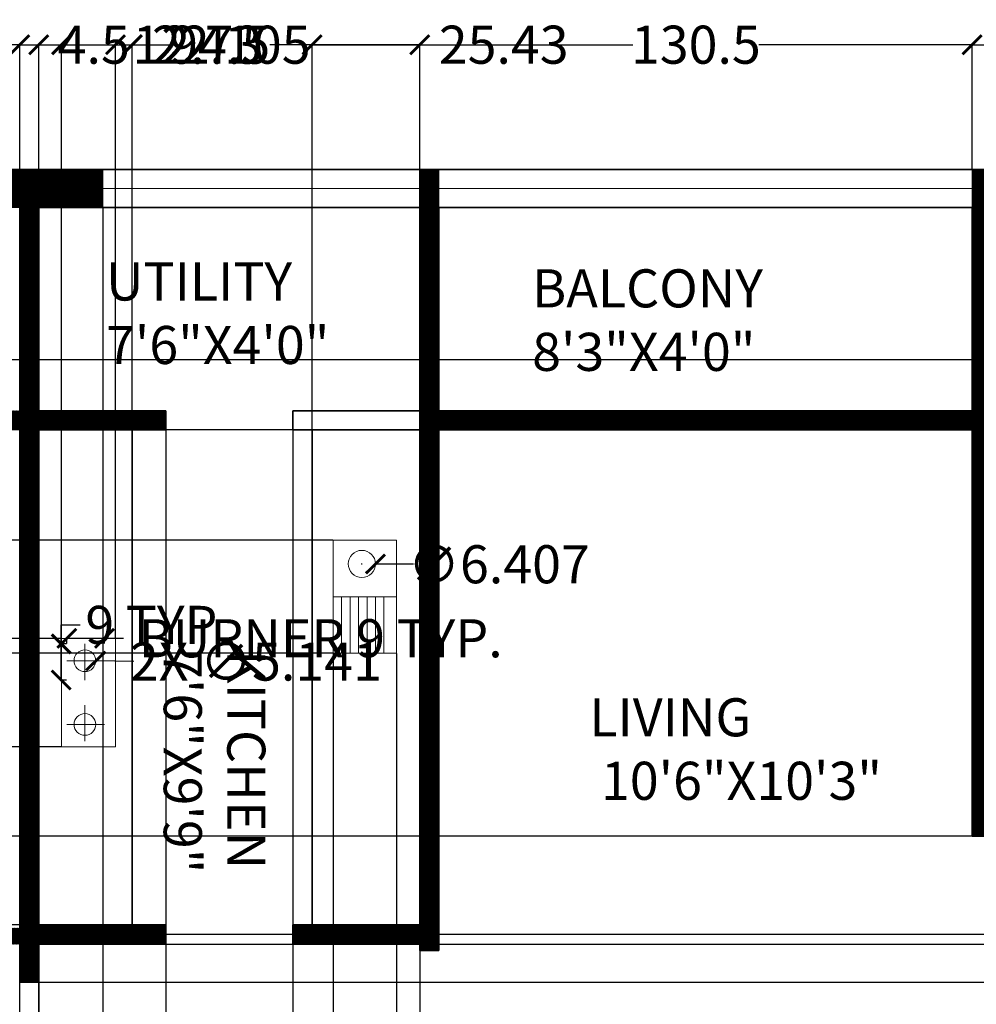
# Model space of a CAD drawing. Units: inches. Extents: x -9 to 675, y 146 to 566.
# Tile 3 of 4: x 192 to 418, y 334 to 566. Entities that reach past the tile are written whole.
import ezdxf

# ---------------------------------------------------------------- set-up
doc = ezdxf.new("R2010")
doc.units = ezdxf.units.IN
doc.header["$MEASUREMENT"] = 0
for name, color, linetype, lineweight in [('A-ANNO-DIMS', 2, 'Continuous', 18), ('A-AREA-IDEN', 7, 'Continuous', 18), ('A-EQPM', 8, 'Continuous', 18), ('A-FLOR-CASE', 8, 'Continuous', 25), ('A-FLOR-FIXT', 9, 'Continuous', 18), ('A-GLAZ', 4, 'Continuous', 18), ('A-WALL', 7, 'Continuous', 35), ('A-WALL-PATT', 252, 'Continuous', 13)]:
    doc.layers.add(name, color=color, linetype=linetype, lineweight=lineweight)
doc.styles.get("Standard").update_dxf_attribs({"font": 'arial.ttf'})
doc.dimstyles.get("Standard").update_dxf_attribs({"dimtxt": 9, "dimasz": 4.5, "dimexe": 0.18, "dimexo": 0.0625, "dimgap": 0.09, "dimtad": 0, "dimtih": 1, "dimtoh": 1, "dimdec": 1, "dimzin": 0, "dimdsep": 46, "dimlunit": 4, "dimtxsty": 'Standard', "dimblk": 'ARCHTICK', "dimcen": 0.09, "dimadec": 0, "dimazin": 0, "dimtfac": 1, "dimtdec": 1, "dimtofl": 0, "dimtmove": 0, "dimatfit": 3, "dimfxl": 1, "dimtolj": 1, "dimtzin": 0, "dimarcsym": 0})

# ---------------------------------------------------------------- blocks, each defined once
blk = doc.blocks.new('COOKTOP-BURNER')
for p, q in [((4.27, 4.56), (4.27, 8.54)), ((4.27, 8.54), (4.27, 4.56)), ((4.27, 4.56), (0, 4.56)), ((4.27, 4.56), (8.88, 4.56)), ((8.88, 4.56), (4.27, 4.56)), ((4.27, 4.56), (4.27, 0)), ((4.27, 0), (4.27, 4.56))]:
    blk.add_line(p, q)
blk.add_circle((4.27, 4.56), 2.57)
blk = doc.blocks.new('_ArchTick')
at = {"color": 0, "linetype": 'ByBlock', "const_width": 0.15}
blk.add_lwpolyline([(-0.5, -0.5), (0.5, 0.5)], dxfattribs=at)
blk = doc.blocks.new('*D6')
at = {"layer": 'A-ANNO-DIMS', "color": 0, "lineweight": -2, "transparency": 16777216}
for p, q in [((203.45, 418.99), (203.45, 420.43)), ((203.45, 420.25), (212.33, 420.25)), ((212.33, 418.99), (212.33, 420.43)), ((212.33, 420.25), (216.83, 420.25))]:
    blk.add_line(p, q, dxfattribs=at)
at = {"layer": 'Defpoints', "color": 0, "transparency": 16777216}
for p in [(203.45, 418.92), (212.33, 420.25), (212.33, 418.92)]:
    blk.add_point(p, dxfattribs=at)
at = {"layer": 'A-ANNO-DIMS', "color": 0, "lineweight": -2, "transparency": 16777216, "xscale": 4.5, "yscale": 4.5, "zscale": 4.5, "rotation": 180}
blk.add_blockref('_ArchTick', (203.45, 420.25), dxfattribs=at)
at = {"layer": 'A-ANNO-DIMS', "color": 0, "lineweight": -2, "transparency": 16777216, "xscale": 4.5, "yscale": 4.5, "zscale": 4.5}
blk.add_blockref('_ArchTick', (212.33, 420.25), dxfattribs=at)
at = {"layer": 'A-ANNO-DIMS', "color": 0, "transparency": 16777216, "insert": (263.42, 420.25), "char_height": 9, "attachment_point": 5}
blk.add_mtext('\\A1;BURNER 9 TYP.', dxfattribs=at)
blk = doc.blocks.new('*D7')
at = {"layer": 'A-ANNO-DIMS', "color": 0, "lineweight": -2, "transparency": 16777216}
for p, q in [((202.12, 418.92), (202.12, 423.42)), ((202.12, 423.42), (206.62, 423.42)), ((203.39, 418.92), (201.94, 418.92)), ((202.12, 410.39), (202.12, 418.92)), ((203.39, 410.39), (201.94, 410.39))]:
    blk.add_line(p, q, dxfattribs=at)
at = {"layer": 'Defpoints', "color": 0, "transparency": 16777216}
for p in [(202.12, 418.92), (203.45, 418.92), (203.45, 410.39)]:
    blk.add_point(p, dxfattribs=at)
at = {"layer": 'A-ANNO-DIMS', "color": 0, "lineweight": -2, "transparency": 16777216, "xscale": 4.5, "yscale": 4.5, "zscale": 4.5}
for p, rotation in [((202.12, 418.92), 90), ((202.12, 410.39), 270)]:
    blk.add_blockref('_ArchTick', p, dxfattribs=dict(at, rotation=rotation))
at = {"layer": 'A-ANNO-DIMS', "color": 0, "transparency": 16777216, "insert": (225.12, 423.42), "char_height": 9, "attachment_point": 5}
blk.add_mtext('\\A1;9 TYP.', dxfattribs=at)
blk = doc.blocks.new('*D11')
at = {"layer": 'A-ANNO-DIMS', "color": 0, "lineweight": -2, "transparency": 16777216}
for p, q in [((121.3, 531.07), (121.3, 560.69)), ((192.3, 522.07), (192.3, 560.69)), ((121.3, 560.51), (151.17, 560.51)), ((192.3, 560.51), (162.43, 560.51))]:
    blk.add_line(p, q, dxfattribs=at)
at = {"layer": 'Defpoints', "color": 0, "transparency": 16777216}
for p in [(192.3, 560.51), (121.3, 531.01), (192.3, 522.01)]:
    blk.add_point(p, dxfattribs=at)
at = {"layer": 'A-ANNO-DIMS', "color": 0, "lineweight": -2, "transparency": 16777216, "xscale": 4.5, "yscale": 4.5, "zscale": 4.5, "rotation": 180}
blk.add_blockref('_ArchTick', (121.3, 560.51), dxfattribs=at)
at = {"layer": 'A-ANNO-DIMS', "color": 0, "lineweight": -2, "transparency": 16777216, "xscale": 4.5, "yscale": 4.5, "zscale": 4.5}
blk.add_blockref('_ArchTick', (192.3, 560.51), dxfattribs=at)
at = {"layer": 'A-ANNO-DIMS', "color": 0, "transparency": 16777216, "insert": (156.8, 560.51), "char_height": 9, "attachment_point": 5}
blk.add_mtext('\\A1;71', dxfattribs=at)
blk = doc.blocks.new('*D12')
at = {"layer": 'A-ANNO-DIMS', "color": 0, "lineweight": -2, "transparency": 16777216}
for p, q in [((192.3, 522.07), (192.3, 560.69)), ((286.8, 531.07), (286.8, 560.69)), ((192.3, 560.51), (227.74, 560.51)), ((286.8, 560.51), (251.37, 560.51))]:
    blk.add_line(p, q, dxfattribs=at)
at = {"layer": 'Defpoints', "color": 0, "transparency": 16777216}
for p in [(286.8, 560.51), (286.8, 531.01), (192.3, 522.01)]:
    blk.add_point(p, dxfattribs=at)
at = {"layer": 'A-ANNO-DIMS', "color": 0, "lineweight": -2, "transparency": 16777216, "xscale": 4.5, "yscale": 4.5, "zscale": 4.5, "rotation": 180}
blk.add_blockref('_ArchTick', (192.3, 560.51), dxfattribs=at)
at = {"layer": 'A-ANNO-DIMS', "color": 0, "lineweight": -2, "transparency": 16777216, "xscale": 4.5, "yscale": 4.5, "zscale": 4.5}
blk.add_blockref('_ArchTick', (286.8, 560.51), dxfattribs=at)
at = {"layer": 'A-ANNO-DIMS', "color": 0, "transparency": 16777216, "insert": (239.55, 560.51), "char_height": 9, "attachment_point": 5}
blk.add_mtext('\\A1;94.5', dxfattribs=at)
blk = doc.blocks.new('*D13')
at = {"layer": 'A-ANNO-DIMS', "color": 0, "lineweight": -2, "transparency": 16777216}
for p, q in [((286.8, 531.07), (286.8, 560.69)), ((417.3, 531.07), (417.3, 560.69)), ((286.8, 560.51), (337.17, 560.51)), ((417.3, 560.51), (366.94, 560.51))]:
    blk.add_line(p, q, dxfattribs=at)
at = {"layer": 'Defpoints', "color": 0, "transparency": 16777216}
for p in [(417.3, 560.51), (286.8, 531.01), (417.3, 531.01)]:
    blk.add_point(p, dxfattribs=at)
at = {"layer": 'A-ANNO-DIMS', "color": 0, "lineweight": -2, "transparency": 16777216, "xscale": 4.5, "yscale": 4.5, "zscale": 4.5, "rotation": 180}
blk.add_blockref('_ArchTick', (286.8, 560.51), dxfattribs=at)
at = {"layer": 'A-ANNO-DIMS', "color": 0, "lineweight": -2, "transparency": 16777216, "xscale": 4.5, "yscale": 4.5, "zscale": 4.5}
blk.add_blockref('_ArchTick', (417.3, 560.51), dxfattribs=at)
at = {"layer": 'A-ANNO-DIMS', "color": 0, "transparency": 16777216, "insert": (352.05, 560.51), "char_height": 9, "attachment_point": 5}
blk.add_mtext('\\A1;130.5', dxfattribs=at)
blk = doc.blocks.new('*D14')
at = {"layer": 'A-ANNO-DIMS', "color": 0, "lineweight": -2, "transparency": 16777216}
for p, q in [((417.3, 531.07), (417.3, 560.69)), ((550.8, 531.07), (550.8, 560.69)), ((417.3, 560.51), (469.17, 560.51)), ((550.8, 560.51), (498.94, 560.51))]:
    blk.add_line(p, q, dxfattribs=at)
at = {"layer": 'Defpoints', "color": 0, "transparency": 16777216}
for p in [(550.8, 560.51), (417.3, 531.01), (550.8, 531.01)]:
    blk.add_point(p, dxfattribs=at)
at = {"layer": 'A-ANNO-DIMS', "color": 0, "lineweight": -2, "transparency": 16777216, "xscale": 4.5, "yscale": 4.5, "zscale": 4.5, "rotation": 180}
blk.add_blockref('_ArchTick', (417.3, 560.51), dxfattribs=at)
at = {"layer": 'A-ANNO-DIMS', "color": 0, "lineweight": -2, "transparency": 16777216, "xscale": 4.5, "yscale": 4.5, "zscale": 4.5}
blk.add_blockref('_ArchTick', (550.8, 560.51), dxfattribs=at)
at = {"layer": 'A-ANNO-DIMS', "color": 0, "transparency": 16777216, "insert": (484.05, 560.51), "char_height": 9, "attachment_point": 5}
blk.add_mtext('\\A1;133.5', dxfattribs=at)
blk = doc.blocks.new('*D26')
at = {"layer": 'A-ANNO-DIMS', "color": 0, "lineweight": -2, "transparency": 16777216}
for p, q in [((211.96, 521.95), (211.96, 151.83)), ((286.8, 521.95), (286.8, 151.83)), ((211.96, 152.01), (234.16, 152.01)), ((286.8, 152.01), (264.6, 152.01))]:
    blk.add_line(p, q, dxfattribs=at)
at = {"layer": 'Defpoints', "color": 0, "transparency": 16777216}
for p in [(211.96, 522.01), (286.8, 522.01), (286.8, 152.01)]:
    blk.add_point(p, dxfattribs=at)
at = {"layer": 'A-ANNO-DIMS', "color": 0, "lineweight": -2, "transparency": 16777216, "xscale": 4.5, "yscale": 4.5, "zscale": 4.5, "rotation": 180}
blk.add_blockref('_ArchTick', (211.96, 152.01), dxfattribs=at)
at = {"layer": 'A-ANNO-DIMS', "color": 0, "lineweight": -2, "transparency": 16777216, "xscale": 4.5, "yscale": 4.5, "zscale": 4.5}
blk.add_blockref('_ArchTick', (286.8, 152.01), dxfattribs=at)
at = {"layer": 'A-ANNO-DIMS', "color": 0, "transparency": 16777216, "insert": (249.38, 152.01), "char_height": 9, "attachment_point": 5}
blk.add_mtext('\\A1;74.84', dxfattribs=at)
blk = doc.blocks.new('*D28')
at = {"layer": 'A-ANNO-DIMS', "color": 0, "lineweight": -2, "transparency": 16777216}
for p, q in [((196.8, 469.45), (196.8, 151.83)), ((226.8, 469.45), (226.8, 151.83)), ((196.8, 152.01), (205.28, 152.01)), ((226.8, 152.01), (218.32, 152.01))]:
    blk.add_line(p, q, dxfattribs=at)
at = {"layer": 'Defpoints', "color": 0, "transparency": 16777216}
for p in [(196.8, 469.51), (226.8, 469.51), (226.8, 152.01)]:
    blk.add_point(p, dxfattribs=at)
at = {"layer": 'A-ANNO-DIMS', "color": 0, "lineweight": -2, "transparency": 16777216, "xscale": 4.5, "yscale": 4.5, "zscale": 4.5, "rotation": 180}
blk.add_blockref('_ArchTick', (196.8, 152.01), dxfattribs=at)
at = {"layer": 'A-ANNO-DIMS', "color": 0, "lineweight": -2, "transparency": 16777216, "xscale": 4.5, "yscale": 4.5, "zscale": 4.5}
blk.add_blockref('_ArchTick', (226.8, 152.01), dxfattribs=at)
at = {"layer": 'A-ANNO-DIMS', "color": 0, "transparency": 16777216, "insert": (211.8, 152.01), "char_height": 9, "attachment_point": 5}
blk.add_mtext('\\A1;30', dxfattribs=at)
blk = doc.blocks.new('*D29')
at = {"layer": 'A-ANNO-DIMS', "color": 0, "lineweight": -2, "transparency": 16777216}
for p, q in [((226.8, 469.45), (226.8, 151.83)), ((256.8, 469.45), (256.8, 151.83)), ((226.8, 152.01), (235.28, 152.01)), ((256.8, 152.01), (248.32, 152.01))]:
    blk.add_line(p, q, dxfattribs=at)
at = {"layer": 'Defpoints', "color": 0, "transparency": 16777216}
for p in [(226.8, 469.51), (256.8, 469.51), (256.8, 152.01)]:
    blk.add_point(p, dxfattribs=at)
at = {"layer": 'A-ANNO-DIMS', "color": 0, "lineweight": -2, "transparency": 16777216, "xscale": 4.5, "yscale": 4.5, "zscale": 4.5, "rotation": 180}
blk.add_blockref('_ArchTick', (226.8, 152.01), dxfattribs=at)
at = {"layer": 'A-ANNO-DIMS', "color": 0, "lineweight": -2, "transparency": 16777216, "xscale": 4.5, "yscale": 4.5, "zscale": 4.5}
blk.add_blockref('_ArchTick', (256.8, 152.01), dxfattribs=at)
at = {"layer": 'A-ANNO-DIMS', "color": 0, "transparency": 16777216, "insert": (241.8, 152.01), "char_height": 9, "attachment_point": 5}
blk.add_mtext('\\A1;30', dxfattribs=at)
blk = doc.blocks.new('*D30')
at = {"layer": 'A-ANNO-DIMS', "color": 0, "lineweight": -2, "transparency": 16777216}
for p, q in [((226.8, 347.95), (226.8, 151.83)), ((256.8, 347.95), (256.8, 151.83)), ((226.8, 152.01), (235.28, 152.01)), ((256.8, 152.01), (248.32, 152.01))]:
    blk.add_line(p, q, dxfattribs=at)
at = {"layer": 'Defpoints', "color": 0, "transparency": 16777216}
for p in [(226.8, 348.01), (256.8, 348.01), (256.8, 152.01)]:
    blk.add_point(p, dxfattribs=at)
at = {"layer": 'A-ANNO-DIMS', "color": 0, "lineweight": -2, "transparency": 16777216, "xscale": 4.5, "yscale": 4.5, "zscale": 4.5, "rotation": 180}
blk.add_blockref('_ArchTick', (226.8, 152.01), dxfattribs=at)
at = {"layer": 'A-ANNO-DIMS', "color": 0, "lineweight": -2, "transparency": 16777216, "xscale": 4.5, "yscale": 4.5, "zscale": 4.5}
blk.add_blockref('_ArchTick', (256.8, 152.01), dxfattribs=at)
at = {"layer": 'A-ANNO-DIMS', "color": 0, "transparency": 16777216, "insert": (241.8, 152.01), "char_height": 9, "attachment_point": 5}
blk.add_mtext('\\A1;30', dxfattribs=at)
blk = doc.blocks.new('*D33')
at = {"layer": 'A-ANNO-DIMS', "color": 0, "lineweight": -2, "transparency": 16777216}
for p, q in [((655.8, 348.01), (655.8, 352.51)), ((655.8, 352.51), (660.3, 352.51)), ((196.87, 348.01), (655.98, 348.01)), ((655.8, 339.01), (655.8, 348.01)), ((196.87, 339.01), (655.98, 339.01))]:
    blk.add_line(p, q, dxfattribs=at)
at = {"layer": 'Defpoints', "color": 0, "transparency": 16777216}
for p in [(196.8, 348.01), (655.8, 348.01), (196.8, 339.01)]:
    blk.add_point(p, dxfattribs=at)
at = {"layer": 'A-ANNO-DIMS', "color": 0, "lineweight": -2, "transparency": 16777216, "xscale": 4.5, "yscale": 4.5, "zscale": 4.5}
for p, rotation in [((655.8, 348.01), 90), ((655.8, 339.01), 270)]:
    blk.add_blockref('_ArchTick', p, dxfattribs=dict(at, rotation=rotation))
at = {"layer": 'A-ANNO-DIMS', "color": 0, "transparency": 16777216, "insert": (663.35, 352.51), "char_height": 9, "attachment_point": 5}
blk.add_mtext('\\A1;9', dxfattribs=at)
blk = doc.blocks.new('*D34')
at = {"layer": 'A-ANNO-DIMS', "color": 0, "lineweight": -2, "transparency": 16777216}
for p, q in [((196.87, 339.01), (655.98, 339.01)), ((655.8, 339.01), (655.8, 322.62)), ((655.8, 297.01), (655.8, 313.4)), ((196.87, 297.01), (655.98, 297.01))]:
    blk.add_line(p, q, dxfattribs=at)
at = {"layer": 'Defpoints', "color": 0, "transparency": 16777216}
for p in [(196.8, 339.01), (655.8, 339.01), (196.8, 297.01)]:
    blk.add_point(p, dxfattribs=at)
at = {"layer": 'A-ANNO-DIMS', "color": 0, "lineweight": -2, "transparency": 16777216, "xscale": 4.5, "yscale": 4.5, "zscale": 4.5}
for p, rotation in [((655.8, 339.01), 90), ((655.8, 297.01), 270)]:
    blk.add_blockref('_ArchTick', p, dxfattribs=dict(at, rotation=rotation))
at = {"layer": 'A-ANNO-DIMS', "color": 0, "transparency": 16777216, "insert": (655.8, 318.01), "char_height": 9, "attachment_point": 5}
blk.add_mtext('\\A1;42', dxfattribs=at)
blk = doc.blocks.new('*D42')
at = {"layer": 'A-ANNO-DIMS', "color": 0, "lineweight": -2, "transparency": 16777216}
for p, q in [((196.8, 352.57), (196.8, 560.69)), ((218.91, 352.57), (218.91, 560.69)), ((196.8, 560.51), (218.91, 560.51)), ((218.91, 560.51), (223.41, 560.51))]:
    blk.add_line(p, q, dxfattribs=at)
at = {"layer": 'Defpoints', "color": 0, "transparency": 16777216}
for p in [(218.91, 560.51), (196.8, 352.51), (218.91, 352.51)]:
    blk.add_point(p, dxfattribs=at)
at = {"layer": 'A-ANNO-DIMS', "color": 0, "lineweight": -2, "transparency": 16777216, "xscale": 4.5, "yscale": 4.5, "zscale": 4.5, "rotation": 180}
blk.add_blockref('_ArchTick', (196.8, 560.51), dxfattribs=at)
at = {"layer": 'A-ANNO-DIMS', "color": 0, "lineweight": -2, "transparency": 16777216, "xscale": 4.5, "yscale": 4.5, "zscale": 4.5}
blk.add_blockref('_ArchTick', (218.91, 560.51), dxfattribs=at)
at = {"layer": 'A-ANNO-DIMS', "color": 0, "transparency": 16777216, "insert": (242.29, 560.51), "char_height": 9, "attachment_point": 5}
blk.add_mtext('\\A1;22.105', dxfattribs=at)
blk = doc.blocks.new('*D43')
at = {"layer": 'A-ANNO-DIMS', "color": 0, "lineweight": -2, "transparency": 16777216}
for p, q in [((261.37, 352.57), (261.37, 560.69)), ((286.8, 352.57), (286.8, 560.69)), ((261.37, 560.51), (286.8, 560.51)), ((286.8, 560.51), (291.3, 560.51))]:
    blk.add_line(p, q, dxfattribs=at)
at = {"layer": 'Defpoints', "color": 0, "transparency": 16777216}
for p in [(286.8, 560.51), (261.37, 352.51), (286.8, 352.51)]:
    blk.add_point(p, dxfattribs=at)
at = {"layer": 'A-ANNO-DIMS', "color": 0, "lineweight": -2, "transparency": 16777216, "xscale": 4.5, "yscale": 4.5, "zscale": 4.5, "rotation": 180}
blk.add_blockref('_ArchTick', (261.37, 560.51), dxfattribs=at)
at = {"layer": 'A-ANNO-DIMS', "color": 0, "lineweight": -2, "transparency": 16777216, "xscale": 4.5, "yscale": 4.5, "zscale": 4.5}
blk.add_blockref('_ArchTick', (286.8, 560.51), dxfattribs=at)
at = {"layer": 'A-ANNO-DIMS', "color": 0, "transparency": 16777216, "insert": (306.65, 560.51), "char_height": 9, "attachment_point": 5}
blk.add_mtext('\\A1;25.43', dxfattribs=at)
blk = doc.blocks.new('*D46')
at = {"layer": 'A-ANNO-DIMS', "color": 0, "lineweight": -2, "transparency": 16777216}
for p, q in [((435.74, 522.01), (9.62, 522.01)), ((9.8, 522.01), (9.8, 508.7)), ((9.8, 486.01), (9.8, 499.32)), ((445.74, 486.01), (9.62, 486.01))]:
    blk.add_line(p, q, dxfattribs=at)
at = {"layer": 'Defpoints', "color": 0, "transparency": 16777216}
for p in [(435.8, 522.01), (9.8, 486.01), (445.8, 486.01)]:
    blk.add_point(p, dxfattribs=at)
at = {"layer": 'A-ANNO-DIMS', "color": 0, "lineweight": -2, "transparency": 16777216, "xscale": 4.5, "yscale": 4.5, "zscale": 4.5}
for p, rotation in [((9.8, 522.01), 90), ((9.8, 486.01), 270)]:
    blk.add_blockref('_ArchTick', p, dxfattribs=dict(at, rotation=rotation))
at = {"layer": 'A-ANNO-DIMS', "color": 0, "transparency": 16777216, "insert": (9.8, 504.01), "char_height": 9, "attachment_point": 5}
blk.add_mtext('\\A1;36', dxfattribs=at)
blk = doc.blocks.new('*D47')
at = {"layer": 'A-ANNO-DIMS', "color": 0, "lineweight": -2, "transparency": 16777216}
for p, q in [((617.24, 373.51), (9.62, 373.51)), ((9.8, 373.51), (9.8, 366.56)), ((9.8, 350.24), (9.8, 357.19)), ((602.52, 350.24), (9.62, 350.24))]:
    blk.add_line(p, q, dxfattribs=at)
at = {"layer": 'Defpoints', "color": 0, "transparency": 16777216}
for p in [(617.3, 373.51), (9.8, 350.24), (602.59, 350.24)]:
    blk.add_point(p, dxfattribs=at)
at = {"layer": 'A-ANNO-DIMS', "color": 0, "lineweight": -2, "transparency": 16777216, "xscale": 4.5, "yscale": 4.5, "zscale": 4.5}
for p, rotation in [((9.8, 373.51), 90), ((9.8, 350.24), 270)]:
    blk.add_blockref('_ArchTick', p, dxfattribs=dict(at, rotation=rotation))
at = {"layer": 'A-ANNO-DIMS', "color": 0, "transparency": 16777216, "insert": (9.8, 361.87), "char_height": 9, "attachment_point": 5}
blk.add_mtext('\\A1;23.27', dxfattribs=at)
blk = doc.blocks.new('*D50')
at = {"layer": 'A-ANNO-DIMS', "color": 0, "lineweight": -2, "transparency": 16777216}
for p, q in [((192.3, 297.07), (192.3, 560.69)), ((196.8, 297.07), (196.8, 560.69)), ((192.3, 560.51), (196.8, 560.51)), ((196.8, 560.51), (201.3, 560.51))]:
    blk.add_line(p, q, dxfattribs=at)
at = {"layer": 'Defpoints', "color": 0, "transparency": 16777216}
for p in [(196.8, 560.51), (192.3, 297.01), (196.8, 297.01)]:
    blk.add_point(p, dxfattribs=at)
at = {"layer": 'A-ANNO-DIMS', "color": 0, "lineweight": -2, "transparency": 16777216, "xscale": 4.5, "yscale": 4.5, "zscale": 4.5, "rotation": 180}
blk.add_blockref('_ArchTick', (192.3, 560.51), dxfattribs=at)
at = {"layer": 'A-ANNO-DIMS', "color": 0, "lineweight": -2, "transparency": 16777216, "xscale": 4.5, "yscale": 4.5, "zscale": 4.5}
blk.add_blockref('_ArchTick', (196.8, 560.51), dxfattribs=at)
at = {"layer": 'A-ANNO-DIMS', "color": 0, "transparency": 16777216, "insert": (209.8, 560.51), "char_height": 9, "attachment_point": 5}
blk.add_mtext('\\A1;4.5', dxfattribs=at)
blk = doc.blocks.new('*D51')
at = {"layer": 'A-ANNO-DIMS', "color": 0, "lineweight": -2, "transparency": 16777216}
for p, q in [((266.36, 416.64), (266.36, 151.83)), ((281.29, 416.64), (281.29, 151.83)), ((266.36, 152.01), (281.29, 152.01)), ((281.29, 152.01), (285.79, 152.01))]:
    blk.add_line(p, q, dxfattribs=at)
at = {"layer": 'Defpoints', "color": 0, "transparency": 16777216}
for p in [(266.36, 416.7), (281.29, 416.7), (281.29, 152.01)]:
    blk.add_point(p, dxfattribs=at)
at = {"layer": 'A-ANNO-DIMS', "color": 0, "lineweight": -2, "transparency": 16777216, "xscale": 4.5, "yscale": 4.5, "zscale": 4.5, "rotation": 180}
blk.add_blockref('_ArchTick', (266.36, 152.01), dxfattribs=at)
at = {"layer": 'A-ANNO-DIMS', "color": 0, "lineweight": -2, "transparency": 16777216, "xscale": 4.5, "yscale": 4.5, "zscale": 4.5}
blk.add_blockref('_ArchTick', (281.29, 152.01), dxfattribs=at)
at = {"layer": 'A-ANNO-DIMS', "color": 0, "transparency": 16777216, "insert": (300.65, 152.01), "char_height": 9, "attachment_point": 5}
blk.add_mtext('\\A1;14.93', dxfattribs=at)
blk = doc.blocks.new('*D52')
at = {"layer": 'A-ANNO-DIMS', "color": 0, "lineweight": -2, "transparency": 16777216}
for p, q in [((266.3, 443.4), (9.62, 443.4)), ((9.8, 443.4), (9.8, 434.74)), ((9.8, 416.7), (9.8, 425.37)), ((266.3, 416.7), (9.62, 416.7))]:
    blk.add_line(p, q, dxfattribs=at)
at = {"layer": 'Defpoints', "color": 0, "transparency": 16777216}
for p in [(9.8, 443.4), (266.36, 443.4), (266.36, 416.7)]:
    blk.add_point(p, dxfattribs=at)
at = {"layer": 'A-ANNO-DIMS', "color": 0, "lineweight": -2, "transparency": 16777216, "xscale": 4.5, "yscale": 4.5, "zscale": 4.5}
for p, rotation in [((9.8, 443.4), 90), ((9.8, 416.7), 270)]:
    blk.add_blockref('_ArchTick', p, dxfattribs=dict(at, rotation=rotation))
at = {"layer": 'A-ANNO-DIMS', "color": 0, "transparency": 16777216, "insert": (9.8, 430.05), "char_height": 9, "attachment_point": 5}
blk.add_mtext('\\A1;26.705', dxfattribs=at)
blk = doc.blocks.new('*D53')
at = {"layer": 'A-ANNO-DIMS', "color": 0, "lineweight": -2, "transparency": 16777216}
for p, q in [((261.31, 469.51), (9.62, 469.51)), ((9.8, 469.51), (9.8, 461.14)), ((9.8, 443.4), (9.8, 451.77)), ((266.3, 443.4), (9.62, 443.4))]:
    blk.add_line(p, q, dxfattribs=at)
at = {"layer": 'Defpoints', "color": 0, "transparency": 16777216}
for p in [(261.37, 469.51), (9.8, 443.4), (266.36, 443.4)]:
    blk.add_point(p, dxfattribs=at)
at = {"layer": 'A-ANNO-DIMS', "color": 0, "lineweight": -2, "transparency": 16777216, "xscale": 4.5, "yscale": 4.5, "zscale": 4.5}
for p, rotation in [((9.8, 469.51), 90), ((9.8, 443.4), 270)]:
    blk.add_blockref('_ArchTick', p, dxfattribs=dict(at, rotation=rotation))
at = {"layer": 'A-ANNO-DIMS', "color": 0, "transparency": 16777216, "insert": (9.8, 456.46), "char_height": 9, "attachment_point": 5}
blk.add_mtext('\\A1;26.106', dxfattribs=at)
blk = doc.blocks.new('*D54')
at = {"layer": 'A-ANNO-DIMS', "color": 0, "lineweight": -2, "transparency": 16777216}
for p, q in [((202.21, 420.27), (202.21, 560.69)), ((214.94, 420.27), (214.94, 560.69)), ((202.21, 560.51), (214.94, 560.51)), ((214.94, 560.51), (219.44, 560.51))]:
    blk.add_line(p, q, dxfattribs=at)
at = {"layer": 'Defpoints', "color": 0, "transparency": 16777216}
for p in [(214.94, 560.51), (202.21, 420.2), (214.94, 420.2)]:
    blk.add_point(p, dxfattribs=at)
at = {"layer": 'A-ANNO-DIMS', "color": 0, "lineweight": -2, "transparency": 16777216, "xscale": 4.5, "yscale": 4.5, "zscale": 4.5, "rotation": 180}
blk.add_blockref('_ArchTick', (202.21, 560.51), dxfattribs=at)
at = {"layer": 'A-ANNO-DIMS', "color": 0, "lineweight": -2, "transparency": 16777216, "xscale": 4.5, "yscale": 4.5, "zscale": 4.5}
blk.add_blockref('_ArchTick', (214.94, 560.51), dxfattribs=at)
at = {"layer": 'A-ANNO-DIMS', "color": 0, "transparency": 16777216, "insert": (234.3, 560.51), "char_height": 9, "attachment_point": 5}
blk.add_mtext('\\A1;12.73', dxfattribs=at)
blk = doc.blocks.new('*D55')
at = {"layer": 'A-ANNO-DIMS', "color": 0, "lineweight": -2, "transparency": 16777216}
for p, q in [((202.15, 420.2), (9.62, 420.2)), ((9.8, 420.2), (9.8, 412.11)), ((9.8, 394.64), (9.8, 402.74)), ((202.15, 394.64), (9.62, 394.64))]:
    blk.add_line(p, q, dxfattribs=at)
at = {"layer": 'Defpoints', "color": 0, "transparency": 16777216}
for p in [(9.8, 420.2), (202.21, 420.2), (202.21, 394.64)]:
    blk.add_point(p, dxfattribs=at)
at = {"layer": 'A-ANNO-DIMS', "color": 0, "lineweight": -2, "transparency": 16777216, "xscale": 4.5, "yscale": 4.5, "zscale": 4.5}
for p, rotation in [((9.8, 420.2), 90), ((9.8, 394.64), 270)]:
    blk.add_blockref('_ArchTick', p, dxfattribs=dict(at, rotation=rotation))
at = {"layer": 'A-ANNO-DIMS', "color": 0, "transparency": 16777216, "insert": (9.8, 407.42), "char_height": 9, "attachment_point": 5}
blk.add_mtext('\\A1;25.57', dxfattribs=at)
blk = doc.blocks.new('*D56')
at = {"layer": 'A-ANNO-DIMS', "color": 0, "lineweight": -2, "transparency": 16777216}
for p, q in [((202.15, 394.64), (9.62, 394.64)), ((9.8, 394.64), (9.8, 378.26)), ((9.8, 352.51), (9.8, 368.89)), ((196.74, 352.51), (9.62, 352.51))]:
    blk.add_line(p, q, dxfattribs=at)
at = {"layer": 'Defpoints', "color": 0, "transparency": 16777216}
for p in [(9.8, 394.64), (202.21, 394.64), (196.8, 352.51)]:
    blk.add_point(p, dxfattribs=at)
at = {"layer": 'A-ANNO-DIMS', "color": 0, "lineweight": -2, "transparency": 16777216, "xscale": 4.5, "yscale": 4.5, "zscale": 4.5}
for p, rotation in [((9.8, 394.64), 90), ((9.8, 352.51), 270)]:
    blk.add_blockref('_ArchTick', p, dxfattribs=dict(at, rotation=rotation))
at = {"layer": 'A-ANNO-DIMS', "color": 0, "transparency": 16777216, "insert": (9.8, 373.57), "char_height": 9, "attachment_point": 5}
blk.add_mtext('\\A1;42.126', dxfattribs=at)
blk = doc.blocks.new('*D58')
at = {"layer": 'A-ANNO-DIMS', "color": 0, "lineweight": -2, "transparency": 16777216}
for p, q in [((273.06, 437.82), (273.24, 437.82)), ((273.15, 437.73), (273.15, 437.91)), ((285.35, 437.74), (276.35, 437.8))]:
    blk.add_line(p, q, dxfattribs=at)
at = {"layer": 'Defpoints', "color": 0, "transparency": 16777216}
for p in [(269.95, 437.84), (276.35, 437.8)]:
    blk.add_point(p, dxfattribs=at)
at = {"layer": 'A-ANNO-DIMS', "color": 0, "lineweight": -2, "transparency": 16777216, "xscale": 4.5, "yscale": 4.5, "zscale": 4.5, "rotation": 179.6150108270535}
blk.add_blockref('_ArchTick', (276.35, 437.8), dxfattribs=at)
at = {"layer": 'A-ANNO-DIMS', "color": 0, "transparency": 16777216, "insert": (305.52, 437.74), "char_height": 9, "attachment_point": 5}
blk.add_mtext('\\A1;∅6.407', dxfattribs=at)
blk = doc.blocks.new('*D59')
at = {"layer": 'A-ANNO-DIMS', "color": 0, "lineweight": -2, "transparency": 16777216}
for p, q in [((207.63, 414.94), (207.81, 414.94)), ((207.72, 414.85), (207.72, 415.03)), ((219.29, 414.75), (210.29, 414.9))]:
    blk.add_line(p, q, dxfattribs=at)
at = {"layer": 'Defpoints', "color": 0, "transparency": 16777216}
for p in [(205.15, 414.99), (210.29, 414.9)]:
    blk.add_point(p, dxfattribs=at)
at = {"layer": 'A-ANNO-DIMS', "color": 0, "lineweight": -2, "transparency": 16777216, "xscale": 4.5, "yscale": 4.5, "zscale": 4.5, "rotation": 179.0165020891146}
blk.add_blockref('_ArchTick', (210.29, 414.9), dxfattribs=at)
at = {"layer": 'A-ANNO-DIMS', "color": 0, "transparency": 16777216, "insert": (248.1, 414.75), "char_height": 9, "attachment_point": 5}
blk.add_mtext('\\A1;2X ∅5.141', dxfattribs=at)

msp = doc.modelspace()

# ---------------------------------------------------------------- hatches: boundary and pattern name
at = {"layer": 'A-WALL-PATT'}
h = msp.add_hatch(dxfattribs=at)
h.set_pattern_fill('ANSI31', color=256)
h.paths.add_polyline_path([(361.8026, 244.5097), (357.3026, 244.5097), (357.3026, 228.4917), (286.8026, 228.4917), (196.8026, 228.4917), (196.8026, 297.0097), (192.3026, 297.0097), (192.3026, 190.5097), (196.8026, 190.5097), (196.8026, 219.4917), (286.8026, 219.4917), (357.3026, 219.4917), (357.3026, 217.5097), (357.3026, 214.9917), (361.8026, 214.9917), (361.8026, 217.5097)])
h.paths.add_polyline_path([(532.6092, 217.5097), (541.8026, 217.5097), (550.8026, 217.5097), (626.3026, 217.5097), (626.3026, 373.5097), (626.3026, 378.0097), (617.3026, 378.0097), (617.3026, 373.5097), (617.3026, 226.5097), (550.8026, 226.5097), (541.8026, 226.5097), (488.3026, 226.5097), (488.3026, 331.0097), (483.8026, 331.0097), (474.8026, 331.0097), (474.8026, 326.5097), (483.8026, 326.5097), (483.8026, 226.5097), (421.8026, 226.5097), (421.8026, 326.5097), (444.8026, 326.5097), (444.8026, 331.0097), (421.8026, 331.0097), (417.3026, 331.0097), (417.3026, 217.5097), (417.3026, 190.5097), (387.6027, 190.5097), (361.8026, 190.5097), (361.8026, 195.0097), (357.3026, 195.0097), (357.3026, 190.5097), (357.3026, 181.5097), (387.6027, 181.5097), (421.8026, 181.5097), (532.6092, 181.5097)])
h.paths.add_polyline_path([(421.8026, 190.5097), (421.8026, 217.5097), (523.6092, 217.5097), (523.6092, 190.5097)], flags=16)
h.paths.add_polyline_path([(550.8026, 378.0097), (550.8026, 531.0097), (525.3955, 531.0097), (525.3955, 522.0097), (541.8026, 522.0097), (541.8026, 378.0097), (472.8026, 378.0097), (472.8026, 373.5097), (483.8026, 373.5097), (488.3026, 373.5097), (541.8026, 373.5097), (550.8026, 373.5097)])
h.paths.add_polyline_path([(130.3026, 469.5097), (146.3026, 469.5097), (146.3026, 474.0097), (130.3026, 474.0097), (130.3026, 522.0097), (143.3026, 522.0097), (143.3026, 531.0097), (121.3026, 531.0097), (121.3026, 351.7597), (121.3026, 348.0097), (130.3026, 348.0097), (139.3026, 348.0097), (139.3026, 351.7597), (130.3026, 351.7597)])
h.paths.add_polyline_path([(211.9624, 531.0097), (179.3026, 531.0097), (179.3026, 522.0097), (192.3026, 522.0097), (192.3026, 474.0097), (176.3026, 474.0097), (176.3026, 469.5097), (192.3026, 469.5097), (192.3026, 351.7597), (169.3026, 351.7597), (169.3026, 348.0097), (192.3026, 348.0097), (192.3026, 339.0097), (196.8026, 339.0097), (196.8026, 348.0097), (226.8026, 348.0097), (226.8026, 352.5097), (196.8026, 352.5097), (196.8026, 469.5097), (226.8026, 469.5097), (226.8026, 474.0097), (196.8026, 474.0097), (196.8026, 522.0097), (211.9624, 522.0097)])
h.paths.add_polyline_path([(291.3026, 522.0097), (291.3026, 531.0097), (286.8026, 531.0097), (286.8026, 522.0097), (286.8026, 352.5097), (256.8026, 352.5097), (256.8026, 348.0097), (286.8026, 348.0097), (286.8026, 346.5097), (291.3026, 346.5097)])
h.paths.add_polyline_path([(417.3026, 474.0097), (291.3026, 474.0097), (291.3026, 469.5097), (417.3026, 469.5097)])
h.paths.add_polyline_path([(421.8026, 522.0097), (435.8002, 522.0097), (435.8002, 531.0097), (417.3026, 531.0097), (417.3026, 522.0097), (417.3026, 373.5097), (421.8026, 373.5097), (430.8026, 373.5097), (430.8026, 378.0097), (421.8026, 378.0097)])
h.paths.add_polyline_path([(48.3026, 348.0097), (48.3026, 351.7597), (39.3026, 351.7597), (39.3026, 348.0097), (39.3026, 181.5097), (121.3026, 181.5097), (196.8026, 181.5097), (196.8026, 190.5097), (192.3026, 190.5097), (121.3026, 190.5097), (48.3026, 190.5097)])

# ---------------------------------------------------------------- linework, layer by layer
at = {"layer": 'A-EQPM'}
for p, q in [((202.2142, 420.205), (214.9443, 420.205)), ((202.2142, 394.6354), (202.2142, 420.205)), ((214.9443, 420.205), (214.9443, 394.6354)), ((214.9443, 394.6354), (202.2142, 394.6354))]:
    msp.add_line(p, q, dxfattribs=at)
at = {"layer": 'A-FLOR-CASE'}
for p, q in [((218.9076, 469.5097), (218.9076, 352.5097)), ((261.3749, 469.5097), (261.3749, 352.5097))]:
    msp.add_line(p, q, dxfattribs=at)
at = {"layer": 'A-FLOR-FIXT'}
for p, q in [((266.363, 443.4042), (281.2941, 443.4042)), ((266.363, 416.6988), (266.363, 443.4042)), ((281.2941, 443.4042), (281.2941, 416.6988)), ((266.363, 430.0515), (281.2941, 430.0515)), ((268.363, 416.6988), (268.363, 430.0515)), ((270.363, 416.6988), (270.363, 430.0515)), ((272.363, 416.6988), (272.363, 430.0515)), ((274.363, 416.6988), (274.363, 430.0515)), ((276.363, 416.6988), (276.363, 430.0515)), ((278.363, 416.6988), (278.363, 430.0515)), ((281.2941, 416.6988), (266.363, 416.6988))]:
    msp.add_line(p, q, dxfattribs=at)
msp.add_circle((273.149, 437.8218), 3.2033, dxfattribs=at)
at = {"layer": 'A-GLAZ'}
for p, q in [((211.9624, 522.0097), (211.9624, 531.0097)), ((286.8026, 522.0097), (286.8026, 531.0097)), ((291.3026, 522.0097), (291.3026, 531.0097)), ((417.3026, 522.0097), (417.3026, 531.0097)), ((211.9624, 526.5097), (286.8026, 526.5097)), ((291.3026, 526.5097), (417.3026, 526.5097))]:
    msp.add_line(p, q, dxfattribs=at)
at = {"layer": 'A-WALL'}
for p, q in [((121.3026, 531.0097), (550.8026, 531.0097)), ((196.8026, 522.0097), (196.8026, 474.0097)), ((196.8026, 522.0097), (286.8026, 522.0097)), ((286.8026, 522.0097), (286.8026, 352.5097)), ((291.3026, 522.0097), (291.3026, 346.5097)), ((291.3026, 522.0097), (417.3026, 522.0097)), ((417.3026, 522.0097), (417.3026, 373.5097)), ((226.8026, 474.0097), (196.8026, 474.0097)), ((226.8026, 474.0097), (226.8026, 469.5097)), ((286.8026, 474.0097), (256.8026, 474.0097)), ((256.8026, 474.0097), (256.8026, 469.5097)), ((291.3026, 474.0097), (417.3026, 474.0097)), ((196.8026, 469.5097), (196.8026, 352.5097)), ((226.8026, 469.5097), (196.8026, 469.5097)), ((286.8026, 469.5097), (256.8026, 469.5097)), ((291.3026, 469.5097), (417.3026, 469.5097)), ((421.8026, 373.5097), (417.3026, 373.5097)), ((226.8026, 352.5097), (196.8026, 352.5097)), ((226.8026, 352.5097), (226.8026, 348.0097)), ((286.8026, 352.5097), (256.8026, 352.5097)), ((256.8026, 352.5097), (256.8026, 348.0097)), ((196.8026, 348.0097), (196.8026, 339.0097)), ((226.8026, 348.0097), (196.8026, 348.0097)), ((286.8026, 348.0097), (256.8026, 348.0097)), ((286.8026, 348.0097), (286.8026, 346.5097)), ((291.3026, 346.5097), (286.8026, 346.5097)), ((192.3026, 339.0097), (196.8026, 339.0097))]:
    msp.add_line(p, q, dxfattribs=at)

# ---------------------------------------------------------------- block references
at = {"layer": 'A-EQPM'}
msp.add_blockref('COOKTOP-BURNER', (203.453, 410.386), dxfattribs=at)
at = {"layer": 'A-EQPM', "extrusion": (0, 0, -1), "zscale": -1, "rotation": 180}
msp.add_blockref('COOKTOP-BURNER', (-203.453, 404.4543), dxfattribs=at)

# ---------------------------------------------------------------- texts
at = {"layer": 'A-AREA-IDEN', "char_height": 9, "attachment_point": 1}
for s, insert in [('UTILITY\\P7\'6"X4\'0"', (212.7053, 509.0573)), ('BALCONY\\P8\'3"X4\'0"', (313.3662, 507.4346)), ('LIVING\\P 10\'6"X10\'3"', (326.8828, 406.0813))]:
    msp.add_mtext_dynamic_manual_height_columns(s, width=552.217276, gutter_width=1, heights=[0], dxfattribs=dict(at, insert=insert))
at = {"layer": 'A-AREA-IDEN', "insert": (250.3368, 417.4647), "char_height": 9, "attachment_point": 1, "rotation": 270}
msp.add_mtext_dynamic_manual_height_columns('KITCHEN\\P7\'6"X9\'9"', width=552.217276, gutter_width=1, heights=[0], dxfattribs=at)

# ---------------------------------------------------------------- dimensions: what is measured, and where the dimension line sits
at = {"layer": 'A-ANNO-DIMS'}
for base, p1, p2, override, picture, middle in [((192.3026, 560.5097), (121.3026, 531.0097), (192.3026, 522.0097), {"dimdec": 0, "dimlfac": 1, "dimrnd": 0, "dimzin": 0, "dimdsep": 46, "dimlunit": 2}, '*D11', (156.8026, 560.5097)), ((286.8026, 560.5097), (192.3026, 522.0097), (286.8026, 531.0097), {"dimdec": 1, "dimlfac": 1, "dimrnd": 0, "dimzin": 0, "dimdsep": 46, "dimlunit": 2}, '*D12', (239.5526, 560.5097)), ((196.8026, 560.5097), (192.3026, 297.0097), (196.8026, 297.0097), {"dimdec": 1, "dimlfac": 1, "dimrnd": 0, "dimzin": 0, "dimdsep": 46, "dimlunit": 2}, '*D50', (209.8002, 560.5097)), ((218.9076, 560.5097), (196.8026, 352.5097), (218.9076, 352.5097), {"dimdec": 3, "dimlfac": 1, "dimrnd": 0, "dimzin": 0, "dimdsep": 46, "dimlunit": 2}, '*D42', (242.2895, 560.5097)), ((214.9443, 560.5097), (202.2142, 420.205), (214.9443, 420.205), {"dimdec": 2, "dimlfac": 1, "dimrnd": 0, "dimzin": 0, "dimdsep": 46, "dimlunit": 2}, '*D54', (234.2959, 560.5097)), ((286.8026, 560.5097), (261.3749, 352.5097), (286.8026, 352.5097), {"dimdec": 2, "dimlfac": 1, "dimrnd": 0, "dimzin": 0, "dimdsep": 46, "dimlunit": 2}, '*D43', (306.6546, 560.5097)), ((417.3026, 560.5097), (286.8026, 531.0097), (417.3026, 531.0097), {"dimdec": 1, "dimlfac": 1, "dimrnd": 0, "dimzin": 0, "dimdsep": 46, "dimlunit": 2}, '*D13', (352.0526, 560.5097)), ((550.8026, 560.5097), (417.3026, 531.0097), (550.8026, 531.0097), {"dimdec": 1, "dimlfac": 1, "dimrnd": 0, "dimzin": 0, "dimdsep": 46, "dimlunit": 2}, '*D14', (484.0526, 560.5097)), ((286.8026, 152.0097), (211.9624, 522.0097), (286.8026, 522.0097), {"dimdec": 2, "dimlfac": 1, "dimrnd": 0, "dimzin": 0, "dimdsep": 46, "dimlunit": 2}, '*D26', (249.3825, 152.0097)), ((226.8026, 152.0097), (196.8026, 469.5097), (226.8026, 469.5097), {"dimdec": 0, "dimlfac": 1, "dimrnd": 0, "dimzin": 0, "dimdsep": 46, "dimlunit": 2}, '*D28', (211.8026, 152.0097)), ((256.8026, 152.0097), (226.8026, 469.5097), (256.8026, 469.5097), {"dimdec": 0, "dimlfac": 1, "dimrnd": 0, "dimzin": 0, "dimdsep": 46, "dimlunit": 2}, '*D29', (241.8026, 152.0097)), ((281.2941, 152.0097), (266.363, 416.6988), (281.2941, 416.6988), {"dimdec": 2, "dimlfac": 1, "dimrnd": 0, "dimzin": 0, "dimdsep": 46, "dimlunit": 2}, '*D51', (300.6457, 152.0097)), ((256.8026, 152.0097), (226.8026, 348.0097), (256.8026, 348.0097), {"dimdec": 0, "dimlfac": 1, "dimrnd": 0, "dimzin": 0, "dimdsep": 46, "dimlunit": 2}, '*D30', (241.8026, 152.0097))]:
    dim = msp.add_linear_dim(base=base, p1=p1, p2=p2, dimstyle='Standard', override=override, dxfattribs=at)
    dim.commit()
    dim.dimension.update_dxf_attribs({"geometry": picture, "text_midpoint": middle})
for base, p1, p2, override, picture, middle in [((9.8026, 486.0097), (435.8002, 522.0097), (445.8026, 486.0097), {"dimdec": 0, "dimlfac": 1, "dimrnd": 0, "dimzin": 0, "dimdsep": 46, "dimlunit": 2}, '*D46', (9.8026, 504.0097)), ((9.80262, 443.40419), (261.37488, 469.50974), (266.36296, 443.40418), {"dimdec": 3, "dimlfac": 1, "dimrnd": 0, "dimzin": 0, "dimdsep": 46, "dimlunit": 2}, '*D53', (9.80262, 456.45696)), ((9.8026, 443.4042), (266.363, 416.6988), (266.363, 443.4042), {"dimdec": 3, "dimlfac": 1, "dimrnd": 0, "dimzin": 0, "dimdsep": 46, "dimlunit": 2}, '*D52', (9.8026, 430.0515)), ((9.8026, 420.205), (202.2142, 394.6354), (202.2142, 420.205), {"dimdec": 2, "dimlfac": 1, "dimrnd": 0, "dimzin": 0, "dimdsep": 46, "dimlunit": 2}, '*D55', (9.8026, 407.4202)), ((9.8026, 394.6354), (196.8026, 352.5097), (202.2142, 394.6354), {"dimdec": 3, "dimlfac": 1, "dimrnd": 0, "dimzin": 0, "dimdsep": 46, "dimlunit": 2}, '*D56', (9.8026, 373.5726)), ((9.8026, 350.2376), (617.3026, 373.5097), (602.5856, 350.2376), {"dimdec": 2, "dimlfac": 1, "dimrnd": 0, "dimzin": 0, "dimdsep": 46, "dimlunit": 2}, '*D47', (9.8026, 361.8737)), ((655.8026, 348.0097), (196.8026, 339.0097), (196.8026, 348.0097), {"dimdec": 0, "dimlfac": 1, "dimrnd": 0, "dimzin": 0, "dimdsep": 46, "dimlunit": 2}, '*D33', (663.3517, 352.5097)), ((655.8026, 339.0097), (196.8026, 297.0097), (196.8026, 339.0097), {"dimdec": 0, "dimlfac": 1, "dimrnd": 0, "dimzin": 0, "dimdsep": 46, "dimlunit": 2}, '*D34', (655.8026, 318.0097))]:
    dim = msp.add_linear_dim(base=base, p1=p1, p2=p2, angle=90, dimstyle='Standard', override=override, dxfattribs=at)
    dim.commit()
    dim.dimension.update_dxf_attribs({"geometry": picture, "text_midpoint": middle})
dim = msp.add_diameter_dim_2p(p1=(269.9457, 437.8434), p2=(276.3522, 437.8003), dimstyle='Standard', override={"dimdec": 3, "dimlfac": 1, "dimrnd": 0, "dimzin": 0, "dimdsep": 46, "dimlunit": 2}, dxfattribs=at)
dim.commit()
dim.dimension.update_dxf_attribs({"geometry": '*D58', "text_midpoint": (285.352, 437.7398), "dimtype": 163})
dim = msp.add_linear_dim(base=(212.3295, 420.2543), p1=(203.4528, 418.9228), p2=(212.3295, 418.9228), text='BURNER <> TYP.', dimstyle='Standard', override={"dimdec": 0, "dimlfac": 1, "dimrnd": 0, "dimzin": 0, "dimdsep": 46, "dimlunit": 2}, dxfattribs=at)
dim.commit()
dim.dimension.update_dxf_attribs({"geometry": '*D6', "text_midpoint": (263.4205, 420.2543)})
dim = msp.add_linear_dim(base=(202.1213, 418.9228), p1=(203.4528, 410.3863), p2=(203.4528, 418.9228), angle=90, text='<> TYP.', dimstyle='Standard', override={"dimdec": 0, "dimlfac": 1, "dimrnd": 0, "dimzin": 0, "dimdsep": 46, "dimlunit": 2}, dxfattribs=at)
dim.commit()
dim.dimension.update_dxf_attribs({"geometry": '*D7', "text_midpoint": (225.1196, 423.4228)})
dim = msp.add_diameter_dim_2p(p1=(205.1523, 414.9884), p2=(210.2925, 414.9001), text='2X <>', dimstyle='Standard', override={"dimdec": 3, "dimlfac": 1, "dimrnd": 0, "dimzin": 0, "dimdsep": 46, "dimlunit": 2}, dxfattribs=at)
dim.commit()
dim.dimension.update_dxf_attribs({"geometry": '*D59', "text_midpoint": (219.2912, 414.7456), "dimtype": 163})

doc.saveas('drawing.dxf')
